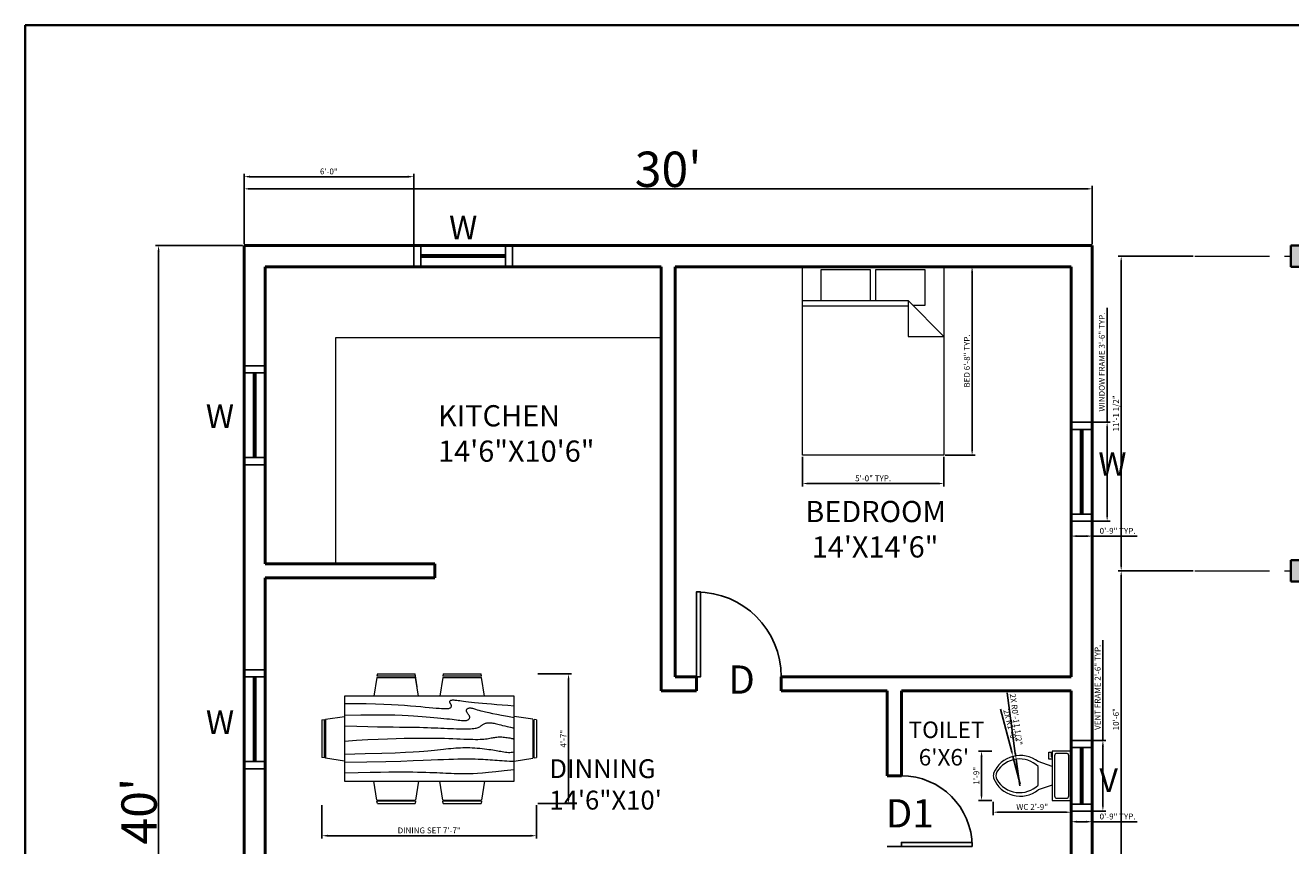
# Model space of a CAD drawing. Units: inches. Extents: x 2150 to 10686, y 1035 to 5077.
# Tile 3 of 12: x 2150 to 2687, y 1753 to 2101. Entities that reach past the tile are written whole.
import ezdxf

# ---------------------------------------------------------------- set-up
doc = ezdxf.new("R2010")
doc.units = ezdxf.units.IN
doc.linetypes.add('CENTER', pattern=[50.8, 31.75, -6.35, 6.35, -6.35])
for name, color, linetype, lineweight in [('A-ANNO-DIMS', 2, 'Continuous', 18), ('A-ANNO-IDEN', 2, 'Continuous', 18), ('A-ANNO-TTLB', 7, 'Continuous', 35), ('A-AREA-IDEN', 7, 'Continuous', 18), ('A-COLS', 7, 'Continuous', 35), ('A-COLS-PATT', 8, 'Continuous', 13), ('A-DOOR', 4, 'Continuous', 25), ('A-FLOR-FIXT', 9, 'Continuous', 18), ('A-FURN', 8, 'Continuous', 18), ('A-GLAZ', 30, 'Continuous', 25), ('A-GRID', 1, 'CENTER', 18), ('A-WALL', 18, 'Continuous', 50)]:
    doc.layers.add(name, color=color, linetype=linetype, lineweight=lineweight)
doc.styles.get("Standard").update_dxf_attribs({"font": 'arial.ttf'})
doc.dimstyles.new('ISO-25', dxfattribs={"dimtxt": 2.5, "dimasz": 2.5, "dimexe": 1.25, "dimexo": 0.625, "dimtad": 1, "dimdec": 0, "dimlunit": 3, "dimtxsty": 'Standard', "dimcen": 2.5, "dimadec": 0, "dimazin": 0, "dimtfac": 1, "dimtdec": 0, "dimtmove": 0, "dimatfit": 3, "dimfxl": 1, "dimarcsym": 0})

# ---------------------------------------------------------------- blocks, each defined once
blk = doc.blocks.new('Bed - Queen')
for p, q in [((0, -80.00003), (0, 0)), ((0, 0), (59.99999, 0)), ((59.99999, 0), (59.99999, -80.00003)), ((7.99999, -1.2), (28.79998, -1.2)), ((7.99999, -14.4), (7.99999, -1.2)), ((28.79998, -1.2), (28.79998, -14.4)), ((31.19999, -1.2), (51.99999, -1.2)), ((31.19999, -14.4), (31.19999, -1.2)), ((51.99999, -1.2), (51.99999, -16.4)), ((0, -14.4), (44.8, -14.4)), ((59.99999, -29.6), (44.8, -14.4)), ((44.8, -14.4), (44.8, -29.6)), ((44.8, -16.8), (0, -16.8)), ((51.99999, -16.4), (46.79936, -16.4)), ((44.8, -29.6), (59.99999, -29.6)), ((59.99999, -80.00003), (0, -80.00003))]:
    blk.add_line(p, q)
blk = doc.blocks.new('Dining Set - 36 x 72 in.')
for p, q in [((-22, 27.5), (-22.1562, 26.50042)), ((-22, 27.5), (-6, 27.5)), ((-5.14035, 21.99844), (-6, 27.5)), ((6, 27.5), (5.8438, 26.50042)), ((6, 27.5), (22, 27.5)), ((22.1563, 26.49966), (22, 27.5)), ((-22.2343, 26.00059), (-23.4847, 17.99762)), ((-22.2304, 26), (-5.7608, 26)), ((-5.8416, 26.5), (-22.1534, 26.5)), ((-4.5152, 17.99762), (-5.7655, 25.99926)), ((5.7657, 26.00059), (4.5153, 17.99762)), ((5.7696, 26), (22.2392, 26)), ((22.1584, 26.5), (5.8466, 26.5)), ((23.4848, 17.99762), (22.2345, 25.99926)), ((36, 18), (-36, 18)), ((-36, 18), (-36, -18)), ((36, -18), (36, 18)), ((-45.5, 8), (-44.5004, 8.15617)), ((-45.5, 8), (-45.5, -8)), ((-44.5, -8.15843), (-44.5, 8.15338)), ((-44.0006, 8.23428), (-35.9976, 9.48474)), ((-44, 8.23041), (-44, -8.23915)), ((44.0006, 8.23428), (35.9976, 9.48474)), ((44, 8.23041), (44, -8.23915)), ((44.5, -8.15843), (44.5, 8.15338)), ((45.5, 8), (44.5005, 8.15617)), ((45.5, 8), (45.5, -8)), ((-44.4997, -8.15631), (-45.5, -8)), ((-35.9976, -9.48476), (-43.9993, -8.2345)), ((35.9976, -9.48476), (43.9993, -8.2345)), ((44.4997, -8.15631), (45.5, -8)), ((-36, -18), (36, -18)), ((-22.2343, -26.0006), (-23.4847, -17.99762)), ((-4.5152, -17.99762), (-5.7655, -25.99928)), ((5.7657, -26.0006), (4.5153, -17.99762)), ((23.4848, -17.99762), (22.2345, -25.99928)), ((-22.2304, -26), (-5.7608, -26)), ((-22, -27.5), (-22.1562, -26.50044)), ((-5.8416, -26.5), (-22.1534, -26.5)), ((-5.8437, -26.49967), (-6, -27.5)), ((5.7696, -26), (22.2392, -26)), ((6, -27.5), (5.8438, -26.50044)), ((22.1584, -26.5), (5.8466, -26.5)), ((22.1563, -26.49967), (22, -27.5)), ((-22, -27.5), (-6, -27.5)), ((6, -27.5), (22, -27.5))]:
    blk.add_line(p, q)
for points in [[(-36, 15), (-31.1772, 14.97754), (-26.8079, 14.91406), (-22.8538, 14.81543), (-19.276, 14.6875), (-16.0362, 14.53613), (-13.0957, 14.36718), (-10.4159, 14.18652), (-7.9583, 14), (-5.6904, 13.81315), (-3.6035, 13.63021), (-1.6954, 13.45508), (0.0365, 13.29166), (1.5945, 13.14388), (2.9811, 13.01562), (4.1988, 12.9108), (5.25, 12.83333), (6.1393, 12.78613), (6.8802, 12.76823), (7.4883, 12.77767), (7.9792, 12.8125), (8.3685, 12.87077), (8.6719, 12.95052), (8.9049, 13.0498), (9.0833, 13.16666), (9.2205, 13.29899), (9.3216, 13.44401), (9.3895, 13.59879), (9.4271, 13.76041), (9.4373, 13.92594), (9.4232, 14.09245), (9.3875, 14.257), (9.3333, 14.41666), (9.2638, 14.56917), (9.1836, 14.71484), (9.0975, 14.85465), (9.0104, 14.98958), (8.9272, 15.1206), (8.8529, 15.2487), (8.7922, 15.37483), (8.75, 15.5), (8.7305, 15.62467), (8.7344, 15.74739), (8.7617, 15.86621), (8.8125, 15.97916), (8.8867, 16.08431), (8.9844, 16.17968), (9.1055, 16.26334), (9.25, 16.33333), (9.4189, 16.38802), (9.6172, 16.42708), (9.8506, 16.45052), (10.125, 16.45833), (10.4463, 16.45052), (10.8203, 16.42708), (11.2529, 16.38802), (11.75, 16.33333), (12.3184, 16.26318), (12.9694, 16.17838), (13.7151, 16.07991), (14.5677, 15.96875), (15.5395, 15.84586), (16.6426, 15.71224), (17.8893, 15.56884), (19.2917, 15.41666), (20.859, 15.25667), (22.5879, 15.08984), (24.4721, 14.91715), (26.5052, 14.73958), (28.6809, 14.5581), (30.9929, 14.3737), (33.4347, 14.18733), (36, 14)], [(-36, 10), (-28.9766, 10.14274), (-23.1725, 10.20442), (-18.4241, 10.19775), (-14.5677, 10.13541), (-11.4399, 10.03011), (-8.877, 9.89453), (-6.7154, 9.74137), (-4.7917, 9.58333), (-2.9698, 9.43082), (-1.2246, 9.28515), (0.4415, 9.14534), (2.026, 9.01041), (3.5266, 8.87939), (4.9408, 8.7513), (6.266, 8.62516), (7.5, 8.5), (8.6411, 8.37549), (9.6914, 8.2539), (10.6538, 8.13818), (11.5312, 8.03125), (12.3267, 7.93603), (13.043, 7.85547), (13.6831, 7.79248), (14.25, 7.75), (14.7471, 7.7303), (15.1797, 7.73307), (15.5537, 7.75732), (15.875, 7.80208), (16.1494, 7.86637), (16.3828, 7.94922), (16.5811, 8.04964), (16.75, 8.16666), (16.8944, 8.29915), (17.0143, 8.44531), (17.1089, 8.60319), (17.1771, 8.77083), (17.218, 8.94629), (17.2305, 9.1276), (17.2137, 9.31282), (17.1667, 9.5), (17.0895, 9.6875), (16.987, 9.875), (16.8649, 10.0625), (16.7292, 10.25), (16.5856, 10.4375), (16.4401, 10.625), (16.2985, 10.8125), (16.1667, 11), (16.05, 11.18733), (15.9518, 11.3737), (15.8752, 11.5581), (15.8229, 11.73958), (15.798, 11.91715), (15.8034, 12.08984), (15.842, 12.25667), (15.9167, 12.41666), (16.0295, 12.56836), (16.1784, 12.70833), (16.3605, 12.83268), (16.5729, 12.9375), (16.8127, 13.01888), (17.0768, 13.07291), (17.3625, 13.0957), (17.6667, 13.08333), (17.9894, 13.03312), (18.3418, 12.94726), (18.7382, 12.82918), (19.1927, 12.68229), (19.7195, 12.51001), (20.3327, 12.31575), (21.0465, 12.10294), (21.875, 11.875), (22.8357, 11.63354), (23.959, 11.37304), (25.2786, 11.08618), (26.8282, 10.76562), (28.6414, 10.40405), (30.752, 9.99414), (33.1936, 9.52856), (36, 9)], [(-36, 5.5), (-30.7157, 5.3348), (-26.069, 5.20963), (-21.9946, 5.11767), (-18.4271, 5.05208), (-15.3009, 5.00602), (-12.5508, 4.97265), (-10.1112, 4.94515), (-7.9167, 4.91666), (-5.909, 4.88167), (-4.0586, 4.83984), (-2.3429, 4.79215), (-0.7396, 4.73958), (0.7739, 4.6831), (2.22, 4.6237), (3.6213, 4.56233), (5, 4.5), (6.373, 4.43782), (7.7344, 4.3776), (9.0723, 4.32129), (10.375, 4.27083), (11.6309, 4.22819), (12.8281, 4.19531), (13.9551, 4.17415), (15, 4.16666), (15.954, 4.17448), (16.819, 4.19791), (17.6001, 4.23698), (18.3021, 4.29166), (18.9299, 4.36198), (19.4883, 4.44791), (19.9823, 4.54948), (20.4167, 4.66666), (20.7969, 4.79899), (21.1302, 4.94401), (21.4245, 5.09879), (21.6875, 5.26041), (21.9271, 5.42594), (22.1511, 5.59245), (22.3672, 5.757), (22.5834, 5.91666), (22.8065, 6.06868), (23.0404, 6.21093), (23.2879, 6.34147), (23.5521, 6.45833), (23.8358, 6.55957), (24.142, 6.64323), (24.4735, 6.70735), (24.8334, 6.75), (25.2235, 6.76969), (25.642, 6.76692), (26.0858, 6.74267), (26.5521, 6.69791), (27.0379, 6.63362), (27.5404, 6.55078), (28.0565, 6.45036), (28.5834, 6.33333), (29.1242, 6.19987), (29.7071, 6.04687), (30.3661, 5.87044), (31.1354, 5.66666), (32.0493, 5.43164), (33.142, 5.16146), (34.4475, 4.85221), (36, 4.5)], [(-36, -1), (-30.7915, -0.6591), (-26.0195, -0.38216), (-21.6519, -0.16284), (-17.6563, 0.00521), (-14.0005, 0.12833), (-10.6523, 0.21289), (-7.5796, 0.26522), (-4.75, 0.29166), (-2.134, 0.29793), (0.2878, 0.28711), (2.5317, 0.26163), (4.6146, 0.22396), (6.5529, 0.17651), (8.3633, 0.12174), (10.0623, 0.06209), (11.6667, 0), (13.1899, -0.06201), (14.6341, -0.1211), (15.9982, -0.17432), (17.2813, -0.21875), (18.4823, -0.25147), (19.6003, -0.26953), (20.6343, -0.27002), (21.5834, -0.25), (22.4481, -0.20768), (23.2357, -0.14584), (23.9549, -0.06836), (24.6146, 0.02083), (25.2235, 0.11784), (25.7904, 0.21875), (26.3241, 0.31966), (26.8334, 0.41666), (27.3265, 0.50618), (27.8099, 0.58593), (28.2894, 0.65397), (28.7709, 0.70833), (29.2601, 0.74707), (29.763, 0.76823), (30.2855, 0.76985), (30.8334, 0.75), (31.4088, 0.70784), (31.9994, 0.64713), (32.589, 0.57275), (33.1615, 0.48958), (33.7008, 0.4025), (34.1908, 0.3164), (34.6153, 0.23616), (34.9584, 0.16666), (35.2099, 0.11165), (35.3848, 0.07031), (35.504, 0.04069), (35.5886, 0.02083), (35.6594, 0.00879), (35.7377, 0.0026), (35.8442, 0.00032), (36, 0)], [(-36, -6.5), (-27.1843, -6.31267), (-20.084, -6.1263), (-14.469, -5.9419), (-10.1094, -5.76042), (-6.7752, -5.58285), (-4.2363, -5.41016), (-2.2629, -5.24333), (-0.625, -5.08334), (0.8708, -4.93099), (2.2715, -4.78646), (3.5872, -4.64974), (4.8281, -4.52084), (6.0046, -4.39974), (7.127, -4.28646), (8.2053, -4.18099), (9.25, -4.08334), (10.2705, -3.99382), (11.2734, -3.91407), (12.2647, -3.84603), (13.25, -3.79167), (14.2354, -3.75293), (15.2266, -3.73177), (16.2295, -3.73015), (17.25, -3.75), (18.2912, -3.79248), (19.3451, -3.85547), (20.4009, -3.93604), (21.4479, -4.03125), (22.4754, -4.13819), (23.4727, -4.25391), (24.4289, -4.37549), (25.3334, -4.5), (26.1785, -4.62492), (26.9694, -4.74935), (27.7145, -4.87281), (28.4219, -4.99479), (29.1, -5.11483), (29.7572, -5.23242), (30.4016, -5.34709), (31.0417, -5.45834), (31.6837, -5.56437), (32.3262, -5.65821), (32.9658, -5.73153), (33.599, -5.77604), (34.2224, -5.78345), (34.8327, -5.74545), (35.4264, -5.65373), (36, -5.5)], [(-36, -10), (-26.4022, -9.81299), (-18.4675, -9.62891), (-11.9839, -9.45069), (-6.7396, -9.28125), (-2.5226, -9.12354), (0.8789, -8.98047), (3.6769, -8.85498), (6.0833, -8.75), (8.2767, -8.66765), (10.3021, -8.60677), (12.1712, -8.56543), (13.8958, -8.54167), (15.4876, -8.53353), (16.9583, -8.53907), (18.3197, -8.55632), (19.5834, -8.58334), (20.7616, -8.61841), (21.8685, -8.66081), (22.9188, -8.71004), (23.9271, -8.76563), (24.9081, -8.82707), (25.8763, -8.89388), (26.8465, -8.96558), (27.8334, -9.04167), (28.8474, -9.12118), (29.8828, -9.20117), (30.93, -9.27824), (31.9792, -9.34896), (33.0205, -9.40991), (34.0443, -9.45768), (35.0407, -9.48885), (36, -9.5)], [(-36, -14.5), (-30.0881, -14.33513), (-25.0332, -14.21224), (-20.7312, -14.12647), (-17.0781, -14.07292), (-13.97, -14.04671), (-11.3027, -14.04297), (-8.9724, -14.05681), (-6.875, -14.08334), (-4.9224, -14.11833), (-3.0905, -14.16016), (-1.3709, -14.20785), (0.2448, -14.26042), (1.7647, -14.3169), (3.1973, -14.3763), (4.5507, -14.43767), (5.8333, -14.5), (7.0554, -14.5621), (8.235, -14.62175), (9.3922, -14.67652), (10.5469, -14.72396), (11.7192, -14.76164), (12.929, -14.78711), (14.1965, -14.79794), (15.5417, -14.79167), (16.9933, -14.76424), (18.6152, -14.70508), (20.4804, -14.60197), (22.6615, -14.44271), (25.2312, -14.21509), (28.2624, -13.9069), (31.8277, -13.50594), (36, -13)]]:
    blk.add_lwpolyline(points)
blk = doc.blocks.new('Toilet - top')
for p, q in [((9.5, -6), (9.5, -2)), ((-10, -8.5), (-8, -8.5)), ((-10, -9.5), (-10, -8.5)), ((-7, -9.5), (-10, -9.5)), ((-8, -8.5), (-8, -8)), ((-7, -8), (-7, -9.5)), ((-4, -8), (-6, -14)), ((4, -8), (6, -14)), ((4, -14), (-4, -14))]:
    blk.add_line(p, q)
blk.add_lwpolyline([(10.5, -8), (10.5, 0), (-10.5, 0), (-10.5, -8)], close=True)
for points in [[(-9.5, -2), (-9.5, -6)], [(8.5, -1), (-8.5, -1)], [(-8.5, -7), (8.5, -7)]]:
    blk.add_lwpolyline(points)
for centre, radius, start, end in [((-8.62, -1.88), 0.884, 81.8699, 188.1301), ((8.62, -1.88), 0.884, 351.8699, 98.1301), ((-8.62, -6.12), 0.884, 171.8699, 278.1301), ((8.62, -6.12), 0.884, 261.8699, 8.1301), ((3.52, -21.58), 12.17, 141.4691, 247.9714), ((4.2, -21.82), 11.33, 136.3677, 238.9468), ((-3.52, -21.58), 12.17, 292.0284, 38.5307), ((-4.2, -21.82), 11.33, 301.053, 43.6321), ((0, -27.88), 4, 245.7318, 294.2682), ((0, -29), 4, 254.8605, 285.1395)]:
    blk.add_arc(centre, radius, start, end)
blk = doc.blocks.new('*U8')
for p, q in [((0, 0), (0, -6)), ((36, 0), (36, -6))]:
    blk.add_line(p, q)
blk.add_lwpolyline([(0, 0), (0, 36), (1.75, 36), (1.75, 0)], close=True)
blk.add_arc((0, 0), 36, 0, 90)
blk = doc.blocks.new('*U10')
for p, q in [((-30, 0), (-30, -6)), ((0, 0), (0, -6))]:
    blk.add_line(p, q)
blk.add_lwpolyline([(0, 0), (0, 30), (-1.75, 30), (-1.75, 0)], close=True)
blk.add_arc((0, 0), 30, 90, 180)
blk = doc.blocks.new('*D12')
at = {"layer": 'A-ANNO-DIMS', "color": 0, "lineweight": -2, "transparency": 16777216}
for p, q in [((2242.69, 2007.92), (2242.69, 2032.59)), ((2245.19, 2031.34), (2600.19, 2031.34)), ((2602.69, 2007.92), (2602.69, 2032.59))]:
    blk.add_line(p, q, dxfattribs=at)
at = {"layer": 'A-ANNO-DIMS', "color": 0, "transparency": 16777216}
for points in [[(2245.19, 2031.76), (2245.19, 2030.92), (2242.69, 2031.34)], [(2600.19, 2031.76), (2600.19, 2030.92), (2602.69, 2031.34)]]:
    blk.add_solid(points, dxfattribs=at)
at = {"layer": 'Defpoints', "color": 0, "transparency": 16777216}
for p in [(2602.69, 2031.34), (2242.69, 2007.29), (2602.69, 2007.29)]:
    blk.add_point(p, dxfattribs=at)
at = {"layer": 'A-ANNO-DIMS', "color": 0, "transparency": 16777216, "insert": (2422.69, 2039.63), "char_height": 2.5, "attachment_point": 5}
blk.add_mtext("{\\H6x;30'}", dxfattribs=at)
blk = doc.blocks.new('*D13')
at = {"layer": 'A-ANNO-DIMS', "color": 0, "lineweight": -2, "transparency": 16777216}
for p, q in [((2242.07, 2007.29), (2205.18, 2007.29)), ((2206.43, 2004.79), (2206.43, 1529.79)), ((2242.07, 1527.29), (2205.18, 1527.29))]:
    blk.add_line(p, q, dxfattribs=at)
at = {"layer": 'A-ANNO-DIMS', "color": 0, "transparency": 16777216}
for points in [[(2206.01, 2004.79), (2206.85, 2004.79), (2206.43, 2007.29)], [(2206.01, 1529.79), (2206.85, 1529.79), (2206.43, 1527.29)]]:
    blk.add_solid(points, dxfattribs=at)
at = {"layer": 'Defpoints', "color": 0, "transparency": 16777216}
for p in [(2242.69, 2007.29), (2206.43, 1527.29), (2242.69, 1527.29)]:
    blk.add_point(p, dxfattribs=at)
at = {"layer": 'A-ANNO-DIMS', "color": 0, "transparency": 16777216, "insert": (2198.15, 1767.29), "char_height": 2.5, "attachment_point": 5, "rotation": 90}
blk.add_mtext("{\\H6x;40'}", dxfattribs=at)
blk = doc.blocks.new('COL-SQUARE-9IN')
for p, q in [((0, 9), (9, 9)), ((0, 0), (0, 9)), ((9, 9), (9, 0)), ((9, 0), (0, 0))]:
    blk.add_line(p, q)
blk = doc.blocks.new('WINDOW-36IN')
for p, q in [((9, 42), (0, 42)), ((9, 39), (0, 39)), ((4, 39), (4, 3)), ((4.5, 39), (4.5, 3)), ((5, 39), (5, 3)), ((9, 3), (0, 3)), ((9, 0), (0, 0))]:
    blk.add_line(p, q)
blk = doc.blocks.new('VENT-24IN')
for p, q in [((0, 30), (9, 30)), ((0, 27), (9, 27)), ((4, 27), (4, 3)), ((4.5, 27), (4.5, 3)), ((5, 27), (5, 3)), ((0, 3), (9, 3)), ((0, 0), (9, 0))]:
    blk.add_line(p, q)
blk = doc.blocks.new('*D40')
at = {"layer": 'A-ANNO-DIMS', "color": 0, "lineweight": -2, "transparency": 16777216}
for p, q in [((2540.32, 1998.29), (2552.94, 1998.29)), ((2551.69, 1920.79), (2551.69, 1995.79)), ((2540.32, 1918.29), (2552.94, 1918.29))]:
    blk.add_line(p, q, dxfattribs=at)
at = {"layer": 'A-ANNO-DIMS', "color": 0, "transparency": 16777216}
for points in [[(2551.28, 1995.79), (2552.11, 1995.79), (2551.69, 1998.29)], [(2551.28, 1920.79), (2552.11, 1920.79), (2551.69, 1918.29)]]:
    blk.add_solid(points, dxfattribs=at)
at = {"layer": 'Defpoints', "color": 0, "transparency": 16777216}
for p in [(2539.69, 1998.29), (2551.69, 1998.29), (2539.69, 1918.29)]:
    blk.add_point(p, dxfattribs=at)
at = {"layer": 'A-ANNO-DIMS', "color": 0, "transparency": 16777216, "insert": (2549.79, 1958.29), "char_height": 2.5, "attachment_point": 5, "rotation": 90}
blk.add_mtext('BED 6\'-8" TYP.', dxfattribs=at)
blk = doc.blocks.new('*D41')
at = {"layer": 'A-ANNO-DIMS', "color": 0, "lineweight": -2, "transparency": 16777216}
for p, q in [((2479.69, 1917.67), (2479.69, 1905.04)), ((2539.69, 1917.67), (2539.69, 1905.04)), ((2482.19, 1906.29), (2537.19, 1906.29))]:
    blk.add_line(p, q, dxfattribs=at)
at = {"layer": 'A-ANNO-DIMS', "color": 0, "transparency": 16777216}
for points in [[(2482.19, 1906.71), (2482.19, 1905.87), (2479.69, 1906.29)], [(2537.19, 1906.71), (2537.19, 1905.87), (2539.69, 1906.29)]]:
    blk.add_solid(points, dxfattribs=at)
at = {"layer": 'Defpoints', "color": 0, "transparency": 16777216}
for p in [(2479.69, 1918.29), (2539.69, 1918.29), (2539.69, 1906.29)]:
    blk.add_point(p, dxfattribs=at)
at = {"layer": 'A-ANNO-DIMS', "color": 0, "transparency": 16777216, "insert": (2509.69, 1908.19), "char_height": 2.5, "attachment_point": 5}
blk.add_mtext('5\'-0" TYP.', dxfattribs=at)
blk = doc.blocks.new('*D44')
at = {"layer": 'A-ANNO-DIMS', "color": 0, "lineweight": -2, "transparency": 16777216}
for p, q in [((2608.99, 1932.29), (2608.99, 1980.87)), ((2603.32, 1932.29), (2610.24, 1932.29)), ((2608.99, 1892.79), (2608.99, 1929.79)), ((2603.32, 1890.29), (2610.24, 1890.29))]:
    blk.add_line(p, q, dxfattribs=at)
at = {"layer": 'A-ANNO-DIMS', "color": 0, "transparency": 16777216}
for points in [[(2608.58, 1929.79), (2609.41, 1929.79), (2608.99, 1932.29)], [(2608.58, 1892.79), (2609.41, 1892.79), (2608.99, 1890.29)]]:
    blk.add_solid(points, dxfattribs=at)
at = {"layer": 'Defpoints', "color": 0, "transparency": 16777216}
for p in [(2602.69, 1932.29), (2608.99, 1932.29), (2602.69, 1890.29)]:
    blk.add_point(p, dxfattribs=at)
at = {"layer": 'A-ANNO-DIMS', "color": 0, "transparency": 16777216, "insert": (2607.07, 1957.83), "char_height": 2.5, "attachment_point": 5, "rotation": 90}
blk.add_mtext('WINDOW FRAME 3\'-6" TYP.', dxfattribs=at)
blk = doc.blocks.new('*D45')
at = {"layer": 'A-ANNO-DIMS', "color": 0, "lineweight": -2, "transparency": 16777216}
for p, q in [((2593.69, 1889.67), (2593.69, 1882.74)), ((2602.69, 1889.67), (2602.69, 1882.74)), ((2596.19, 1883.99), (2600.19, 1883.99)), ((2602.69, 1883.99), (2621.68, 1883.99))]:
    blk.add_line(p, q, dxfattribs=at)
at = {"layer": 'A-ANNO-DIMS', "color": 0, "transparency": 16777216}
for points in [[(2596.19, 1884.41), (2596.19, 1883.57), (2593.69, 1883.99)], [(2600.19, 1884.41), (2600.19, 1883.57), (2602.69, 1883.99)]]:
    blk.add_solid(points, dxfattribs=at)
at = {"layer": 'Defpoints', "color": 0, "transparency": 16777216}
for p in [(2593.69, 1890.29), (2602.69, 1890.29), (2602.69, 1883.99)]:
    blk.add_point(p, dxfattribs=at)
at = {"layer": 'A-ANNO-DIMS', "color": 0, "transparency": 16777216, "insert": (2613.44, 1885.89), "char_height": 2.5, "attachment_point": 5}
blk.add_mtext('0\'-9" TYP.', dxfattribs=at)
blk = doc.blocks.new('*D46')
at = {"layer": 'A-ANNO-DIMS', "color": 0, "lineweight": -2, "transparency": 16777216}
for p, q in [((2607.19, 1797.29), (2607.19, 1839.89)), ((2603.32, 1797.29), (2608.44, 1797.29)), ((2607.19, 1769.79), (2607.19, 1794.79)), ((2603.32, 1767.29), (2608.44, 1767.29))]:
    blk.add_line(p, q, dxfattribs=at)
at = {"layer": 'A-ANNO-DIMS', "color": 0, "transparency": 16777216}
for points in [[(2606.78, 1794.79), (2607.61, 1794.79), (2607.19, 1797.29)], [(2606.78, 1769.79), (2607.61, 1769.79), (2607.19, 1767.29)]]:
    blk.add_solid(points, dxfattribs=at)
at = {"layer": 'Defpoints', "color": 0, "transparency": 16777216}
for p in [(2602.69, 1797.29), (2607.19, 1797.29), (2602.69, 1767.29)]:
    blk.add_point(p, dxfattribs=at)
at = {"layer": 'A-ANNO-DIMS', "color": 0, "transparency": 16777216, "insert": (2605.29, 1819.84), "char_height": 2.5, "attachment_point": 5, "rotation": 90}
blk.add_mtext('VENT FRAME 2\'-6" TYP.', dxfattribs=at)
blk = doc.blocks.new('*D47')
at = {"layer": 'A-ANNO-DIMS', "color": 0, "lineweight": -2, "transparency": 16777216}
for p, q in [((2593.69, 1766.67), (2593.69, 1761.54)), ((2596.19, 1762.79), (2600.19, 1762.79)), ((2602.69, 1766.67), (2602.69, 1761.54)), ((2602.69, 1762.79), (2621.68, 1762.79))]:
    blk.add_line(p, q, dxfattribs=at)
at = {"layer": 'A-ANNO-DIMS', "color": 0, "transparency": 16777216}
for points in [[(2596.19, 1763.21), (2596.19, 1762.37), (2593.69, 1762.79)], [(2600.19, 1763.21), (2600.19, 1762.37), (2602.69, 1762.79)]]:
    blk.add_solid(points, dxfattribs=at)
at = {"layer": 'Defpoints', "color": 0, "transparency": 16777216}
for p in [(2593.69, 1767.29), (2602.69, 1767.29), (2602.69, 1762.79)]:
    blk.add_point(p, dxfattribs=at)
at = {"layer": 'A-ANNO-DIMS', "color": 0, "transparency": 16777216, "insert": (2613.44, 1764.69), "char_height": 2.5, "attachment_point": 5}
blk.add_mtext('0\'-9" TYP.', dxfattribs=at)
blk = doc.blocks.new('*D54')
at = {"layer": 'A-ANNO-DIMS', "color": 0, "lineweight": -2, "transparency": 16777216}
for p, q in [((2560.65, 1771.17), (2560.65, 1765.58)), ((2593.69, 1771.17), (2593.69, 1765.58)), ((2563.15, 1766.83), (2591.19, 1766.83))]:
    blk.add_line(p, q, dxfattribs=at)
at = {"layer": 'A-ANNO-DIMS', "color": 0, "transparency": 16777216}
for points in [[(2563.15, 1767.25), (2563.15, 1766.42), (2560.65, 1766.83)], [(2591.19, 1767.25), (2591.19, 1766.42), (2593.69, 1766.83)]]:
    blk.add_solid(points, dxfattribs=at)
at = {"layer": 'Defpoints', "color": 0, "transparency": 16777216}
for p in [(2560.65, 1771.79), (2593.69, 1771.79), (2593.69, 1766.83)]:
    blk.add_point(p, dxfattribs=at)
at = {"layer": 'A-ANNO-DIMS', "color": 0, "transparency": 16777216, "insert": (2577.17, 1768.75), "char_height": 2.5, "attachment_point": 5}
blk.add_mtext('WC 2\'-9"', dxfattribs=at)
blk = doc.blocks.new('*D55')
at = {"layer": 'A-ANNO-DIMS', "color": 0, "lineweight": -2, "transparency": 16777216}
for p, q in [((2560.02, 1792.79), (2554.44, 1792.79)), ((2555.69, 1790.29), (2555.69, 1774.29)), ((2560.02, 1771.79), (2554.44, 1771.79))]:
    blk.add_line(p, q, dxfattribs=at)
at = {"layer": 'A-ANNO-DIMS', "color": 0, "transparency": 16777216}
for points in [[(2555.27, 1790.29), (2556.11, 1790.29), (2555.69, 1792.79)], [(2555.27, 1774.29), (2556.11, 1774.29), (2555.69, 1771.79)]]:
    blk.add_solid(points, dxfattribs=at)
at = {"layer": 'Defpoints', "color": 0, "transparency": 16777216}
for p in [(2560.65, 1792.79), (2555.69, 1771.79), (2560.65, 1771.79)]:
    blk.add_point(p, dxfattribs=at)
at = {"layer": 'A-ANNO-DIMS', "color": 0, "transparency": 16777216, "insert": (2553.79, 1782.29), "char_height": 2.5, "attachment_point": 5, "rotation": 90}
blk.add_mtext('1\'-9"', dxfattribs=at)
blk = doc.blocks.new('*D56')
at = {"layer": 'A-ANNO-DIMS', "color": 0, "lineweight": -2, "transparency": 16777216}
for p, q in [((2275.77, 1769.89), (2275.77, 1755.61)), ((2366.77, 1769.89), (2366.77, 1755.61)), ((2278.27, 1756.86), (2364.27, 1756.86))]:
    blk.add_line(p, q, dxfattribs=at)
at = {"layer": 'A-ANNO-DIMS', "color": 0, "transparency": 16777216}
for points in [[(2278.27, 1757.28), (2278.27, 1756.44), (2275.77, 1756.86)], [(2364.27, 1757.28), (2364.27, 1756.44), (2366.77, 1756.86)]]:
    blk.add_solid(points, dxfattribs=at)
at = {"layer": 'Defpoints', "color": 0, "transparency": 16777216}
for p in [(2275.77, 1770.51), (2366.77, 1770.51), (2366.77, 1756.86)]:
    blk.add_point(p, dxfattribs=at)
at = {"layer": 'A-ANNO-DIMS', "color": 0, "transparency": 16777216, "insert": (2321.27, 1758.78), "char_height": 2.5, "attachment_point": 5}
blk.add_mtext('DINING SET 7\'-7"', dxfattribs=at)
blk = doc.blocks.new('*D57')
at = {"layer": 'A-ANNO-DIMS', "color": 0, "lineweight": -2, "transparency": 16777216}
for p, q in [((2367.39, 1825.51), (2381.67, 1825.51)), ((2380.42, 1773.01), (2380.42, 1823.01)), ((2367.39, 1770.51), (2381.67, 1770.51))]:
    blk.add_line(p, q, dxfattribs=at)
at = {"layer": 'A-ANNO-DIMS', "color": 0, "transparency": 16777216}
for points in [[(2380, 1823.01), (2380.84, 1823.01), (2380.42, 1825.51)], [(2380, 1773.01), (2380.84, 1773.01), (2380.42, 1770.51)]]:
    blk.add_solid(points, dxfattribs=at)
at = {"layer": 'Defpoints', "color": 0, "transparency": 16777216}
for p in [(2366.77, 1825.51), (2380.42, 1825.51), (2366.77, 1770.51)]:
    blk.add_point(p, dxfattribs=at)
at = {"layer": 'A-ANNO-DIMS', "color": 0, "transparency": 16777216, "insert": (2378.54, 1798.01), "char_height": 2.5, "attachment_point": 5, "rotation": 90}
blk.add_mtext('4\'-7"', dxfattribs=at)
blk = doc.blocks.new('*D80')
at = {"layer": 'A-ANNO-DIMS', "color": 0, "lineweight": -2, "transparency": 16777216}
for p, q in [((2645.54, 2002.79), (2613.71, 2002.79)), ((2614.96, 2000.29), (2614.96, 1871.79)), ((2645.54, 1869.29), (2613.71, 1869.29))]:
    blk.add_line(p, q, dxfattribs=at)
at = {"layer": 'A-ANNO-DIMS', "color": 0, "transparency": 16777216}
for points in [[(2614.55, 2000.29), (2615.38, 2000.29), (2614.96, 2002.79)], [(2614.55, 1871.79), (2615.38, 1871.79), (2614.96, 1869.29)]]:
    blk.add_solid(points, dxfattribs=at)
at = {"layer": 'Defpoints', "color": 0, "transparency": 16777216}
for p in [(2646.16, 2002.79), (2614.96, 1869.29), (2646.16, 1869.29)]:
    blk.add_point(p, dxfattribs=at)
at = {"layer": 'A-ANNO-DIMS', "color": 0, "transparency": 16777216, "insert": (2613.05, 1936.04), "char_height": 2.5, "attachment_point": 5, "rotation": 90}
blk.add_mtext('11\'-1 1/2"', dxfattribs=at)
blk = doc.blocks.new('*D81')
at = {"layer": 'A-ANNO-DIMS', "color": 0, "lineweight": -2, "transparency": 16777216}
for p, q in [((2645.54, 1869.29), (2613.71, 1869.29)), ((2614.96, 1866.79), (2614.96, 1745.79)), ((2645.54, 1743.29), (2613.71, 1743.29))]:
    blk.add_line(p, q, dxfattribs=at)
at = {"layer": 'A-ANNO-DIMS', "color": 0, "transparency": 16777216}
for points in [[(2614.55, 1866.79), (2615.38, 1866.79), (2614.96, 1869.29)], [(2614.55, 1745.79), (2615.38, 1745.79), (2614.96, 1743.29)]]:
    blk.add_solid(points, dxfattribs=at)
at = {"layer": 'Defpoints', "color": 0, "transparency": 16777216}
for p in [(2646.16, 1869.29), (2614.96, 1743.29), (2646.16, 1743.29)]:
    blk.add_point(p, dxfattribs=at)
at = {"layer": 'A-ANNO-DIMS', "color": 0, "transparency": 16777216, "insert": (2613.06, 1806.29), "char_height": 2.5, "attachment_point": 5, "rotation": 90}
blk.add_mtext('10\'-6"', dxfattribs=at)
blk = doc.blocks.new('*D138')
at = {"layer": 'A-ANNO-DIMS', "color": 0, "lineweight": -2, "transparency": 16777216}
for p, q in [((2242.69, 2007.92), (2242.69, 2037.74)), ((2245.19, 2036.49), (2312.19, 2036.49)), ((2314.69, 2007.92), (2314.69, 2037.74))]:
    blk.add_line(p, q, dxfattribs=at)
at = {"layer": 'A-ANNO-DIMS', "color": 0, "transparency": 16777216}
for points in [[(2245.19, 2036.91), (2245.19, 2036.07), (2242.69, 2036.49)], [(2312.19, 2036.91), (2312.19, 2036.07), (2314.69, 2036.49)]]:
    blk.add_solid(points, dxfattribs=at)
at = {"layer": 'Defpoints', "color": 0, "transparency": 16777216}
for p in [(2314.69, 2036.49), (2242.69, 2007.29), (2314.69, 2007.29)]:
    blk.add_point(p, dxfattribs=at)
at = {"layer": 'A-ANNO-DIMS', "color": 0, "transparency": 16777216, "insert": (2278.69, 2038.39), "char_height": 2.5, "attachment_point": 5}
blk.add_mtext('6\'-0"', dxfattribs=at)
blk = doc.blocks.new('*D151')
at = {"layer": 'A-ANNO-DIMS', "color": 0, "lineweight": -2, "transparency": 16777216}
for p, q in [((2563.76, 1810.56), (2568.39, 1792.96)), ((2572.11, 1778.77), (2569.02, 1790.54))]:
    blk.add_line(p, q, dxfattribs=at)
at = {"layer": 'A-ANNO-DIMS', "color": 0, "transparency": 16777216}
blk.add_solid([(2568.79, 1793.07), (2567.98, 1792.85), (2569.02, 1790.54)], dxfattribs=at)
at = {"layer": 'Defpoints', "color": 0, "transparency": 16777216}
for p in [(2569.02, 1790.54), (2572.11, 1778.77)]:
    blk.add_point(p, dxfattribs=at)
at = {"layer": 'A-ANNO-DIMS', "color": 0, "transparency": 16777216, "insert": (2567.59, 1803.45), "char_height": 2.5, "attachment_point": 5, "rotation": 284.7226}
blk.add_mtext('2X R1\'-0"', dxfattribs=at)
blk = doc.blocks.new('*D152')
at = {"layer": 'A-ANNO-DIMS', "color": 0, "lineweight": -2, "transparency": 16777216}
for p, q in [((2566.57, 1817.54), (2570.03, 1791.8)), ((2571.88, 1778.09), (2570.37, 1789.32))]:
    blk.add_line(p, q, dxfattribs=at)
at = {"layer": 'A-ANNO-DIMS', "color": 0, "transparency": 16777216}
blk.add_solid([(2570.45, 1791.85), (2569.62, 1791.74), (2570.37, 1789.32)], dxfattribs=at)
at = {"layer": 'Defpoints', "color": 0, "transparency": 16777216}
for p in [(2570.37, 1789.32), (2571.88, 1778.09)]:
    blk.add_point(p, dxfattribs=at)
at = {"layer": 'A-ANNO-DIMS', "color": 0, "transparency": 16777216, "insert": (2570.04, 1806.16), "char_height": 2.5, "attachment_point": 5, "rotation": 277.658}
blk.add_mtext('2X R0\'-11 1/2"', dxfattribs=at)

msp = doc.modelspace()

# ---------------------------------------------------------------- hatches: boundary and pattern name
at = {"layer": 'A-COLS-PATT'}
h = msp.add_hatch(color=256, dxfattribs=at)
h.dxf.hatch_style = 1
h.paths.add_polyline_path([(2695.9, 2007.29), (2686.9, 2007.29), (2686.9, 1998.29), (2695.9, 1998.29)])
h.paths.add_polyline_path([(2871.4, 2007.29), (2862.4, 2007.29), (2862.4, 1998.29), (2871.4, 1998.29)])
h.paths.add_polyline_path([(3046.9, 2007.29), (3037.9, 2007.29), (3037.9, 1998.29), (3046.9, 1998.29)])
h.paths.add_polyline_path([(2695.9, 1873.79), (2686.9, 1873.79), (2686.9, 1864.79), (2695.9, 1864.79)])
h.paths.add_polyline_path([(2871.4, 1873.79), (2862.4, 1873.79), (2862.4, 1864.79), (2871.4, 1864.79)])
h.paths.add_polyline_path([(3046.9, 1873.79), (3037.9, 1873.79), (3037.9, 1864.79), (3046.9, 1864.79)])
h.paths.add_polyline_path([(2695.9, 1747.79), (2686.9, 1747.79), (2686.9, 1738.79), (2695.9, 1738.79)])
h.paths.add_polyline_path([(2871.4, 1747.79), (2862.4, 1747.79), (2862.4, 1738.79), (2871.4, 1738.79)])
h.paths.add_polyline_path([(3046.9, 1747.79), (3037.9, 1747.79), (3037.9, 1738.79), (3046.9, 1738.79)])
h.paths.add_polyline_path([(2695.9, 1621.79), (2686.9, 1621.79), (2686.9, 1612.79), (2695.9, 1612.79)])
h.paths.add_polyline_path([(2871.4, 1621.79), (2862.4, 1621.79), (2862.4, 1612.79), (2871.4, 1612.79)])
h.paths.add_polyline_path([(3046.9, 1621.79), (3037.9, 1621.79), (3037.9, 1612.79), (3046.9, 1612.79)])
h.paths.add_polyline_path([(2695.9, 1536.29), (2686.9, 1536.29), (2686.9, 1527.29), (2695.9, 1527.29)])
h.paths.add_polyline_path([(2871.4, 1536.29), (2862.4, 1536.29), (2862.4, 1527.29), (2871.4, 1527.29)])
h.paths.add_polyline_path([(3046.9, 1536.29), (3037.9, 1536.29), (3037.9, 1527.29), (3046.9, 1527.29)])

# ---------------------------------------------------------------- linework, layer by layer
at = {"layer": 'A-ANNO-TTLB'}
msp.add_lwpolyline([(2149.86, 2100.72), (3159.01, 2100.72), (3159.01, 1034.91), (2149.86, 1034.91)], close=True, dxfattribs=at)
at = {"layer": 'A-FLOR-FIXT'}
for p, q in [((2281.69, 1872.29), (2281.69, 1968.29)), ((2281.69, 1968.29), (2419.69, 1968.29))]:
    msp.add_line(p, q, dxfattribs=at)
at = {"layer": 'A-GRID'}
for p, q in [((2646.16, 2002.79), (2686.9, 2002.79)), ((2646.16, 1869.29), (2686.9, 1869.29))]:
    msp.add_line(p, q, dxfattribs=at)
at = {"layer": 'A-WALL'}
for p, q in [((2242.69, 2007.29), (2602.69, 2007.29)), ((2242.69, 1527.29), (2242.69, 2007.29)), ((2602.69, 2007.29), (2602.69, 1527.29)), ((2251.69, 1998.29), (2419.69, 1998.29)), ((2251.69, 1872.29), (2251.69, 1998.29)), ((2419.69, 1818.29), (2419.69, 1998.29)), ((2425.69, 1824.29), (2425.69, 1998.29)), ((2425.69, 1998.29), (2593.69, 1998.29)), ((2593.69, 1998.29), (2593.69, 1824.29)), ((2251.69, 1872.29), (2323.69, 1872.29)), ((2323.69, 1866.29), (2323.69, 1872.29)), ((2251.69, 1866.29), (2323.69, 1866.29)), ((2251.69, 1746.29), (2251.69, 1866.29)), ((2425.69, 1824.29), (2434.69, 1824.29)), ((2434.69, 1818.29), (2434.69, 1824.29)), ((2470.69, 1818.29), (2470.69, 1824.29)), ((2470.69, 1824.29), (2593.69, 1824.29)), ((2419.69, 1818.29), (2434.69, 1818.29)), ((2470.69, 1818.29), (2515.69, 1818.29)), ((2515.69, 1818.29), (2515.69, 1782.29)), ((2521.69, 1818.29), (2521.69, 1782.29)), ((2521.69, 1818.29), (2593.69, 1818.29)), ((2593.69, 1818.29), (2593.69, 1746.29)), ((2515.69, 1782.29), (2521.69, 1782.29))]:
    msp.add_line(p, q, dxfattribs=at)

# ---------------------------------------------------------------- block references
at = {"layer": 'A-COLS'}
for p in [(2686.9, 1998.29), (2686.9, 1864.79)]:
    msp.add_blockref('COL-SQUARE-9IN', p, dxfattribs=at)
at = {"layer": 'A-DOOR'}
msp.add_blockref('*U8', (2434.69, 1824.29), dxfattribs=at)
at = {"layer": 'A-DOOR', "rotation": 270}
msp.add_blockref('*U10', (2521.69, 1752.29), dxfattribs=at)
at = {"layer": 'A-FLOR-FIXT', "rotation": 270}
msp.add_blockref('Toilet - top', (2593.69, 1782.29), dxfattribs=at)
at = {"layer": 'A-FURN'}
for name, p in [('Bed - Queen', (2479.69, 1998.29)), ('Dining Set - 36 x 72 in.', (2321.27, 1798.01))]:
    msp.add_blockref(name, p, dxfattribs=at)
at = {"layer": 'A-GLAZ', "rotation": 269.9999999999994}
msp.add_blockref('WINDOW-36IN', (2314.69, 2007.29), dxfattribs=at)
at = {"layer": 'A-GLAZ'}
for name, p in [('WINDOW-36IN', (2242.69, 1914.29)), ('WINDOW-36IN', (2593.69, 1890.29)), ('WINDOW-36IN', (2242.69, 1785.29)), ('VENT-24IN', (2593.69, 1767.29))]:
    msp.add_blockref(name, p, dxfattribs=at)

# ---------------------------------------------------------------- texts
at = {"layer": 'A-ANNO-IDEN', "attachment_point": 1}
for s, width, insert, char_height in [('W', 198.2229, (2329.72, 2019.89), 10), ('W', 198.2229, (2226.47, 1939.91), 10), ('W', 198.2229, (2605.26, 1919.6), 10), ('D', 907.773, (2448.22, 1829.11), 12), ('W', 198.2229, (2226.51, 1810.03), 10), ('V', 198.2229, (2605.72, 1785.42), 10), ('D1', 907.773, (2515.03, 1772.36), 12)]:
    msp.add_mtext_dynamic_manual_height_columns(s, width=width, gutter_width=12.5, heights=[0], dxfattribs=dict(at, insert=insert, char_height=char_height))
at = {"layer": 'A-AREA-IDEN', "attachment_point": 1}
for s, width, insert, char_height in [('KITCHEN\\P14\'6"X10\'6"', 274.4742, (2325.04, 1939.54), 9), ('BEDROOM\\P 14\'X14\'6"', 318.868, (2480.88, 1898.91), 9), ("TOILET\\P  6'X6'", 287.2446, (2524.77, 1805.31), 7), ('DINNING\\P14\'6"X10\'', 560.271, (2372.25, 1789.3), 8)]:
    msp.add_mtext_dynamic_manual_height_columns(s, width=width, gutter_width=12.5, heights=[0], dxfattribs=dict(at, insert=insert, char_height=char_height))

# ---------------------------------------------------------------- dimensions: what is measured, and where the dimension line sits
at = {"layer": 'A-ANNO-DIMS'}
dim = msp.add_linear_dim(base=(2602.69, 2031.34), p1=(2242.69, 2007.29), p2=(2602.69, 2007.29), text='{\\H6x;<>}', dimstyle='ISO-25', override={"dimclrd": 0, "dimclre": 0, "dimclrt": 0}, dxfattribs=at)
dim.commit()
dim.dimension.update_dxf_attribs({"geometry": '*D12', "text_midpoint": (2422.69, 2031.34), "dimtype": 160})
dim = msp.add_linear_dim(base=(2314.69, 2036.49), p1=(2242.69, 2007.29), p2=(2314.69, 2007.29), dimstyle='ISO-25', override={"dimdec": 1, "dimlfac": 1, "dimrnd": 0, "dimzin": 1, "dimdsep": 46, "dimlunit": 4, "dimfrac": 2}, dxfattribs=at)
dim.commit()
dim.dimension.update_dxf_attribs({"geometry": '*D138', "text_midpoint": (2278.69, 2038.39)})
for base, p1, p2, text, override, picture, middle in [((2206.43, 1527.29), (2242.69, 2007.29), (2242.69, 1527.29), '{\\H6x;<>}', {"dimclrd": 0, "dimclre": 0, "dimclrt": 0}, '*D13', (2198.15, 1767.29)), ((2551.69, 1998.29), (2539.69, 1918.29), (2539.69, 1998.29), 'BED <> TYP.', {"dimdec": 1, "dimlfac": 1, "dimrnd": 0, "dimzin": 1, "dimdsep": 46, "dimlunit": 4, "dimfrac": 2}, '*D40', (2549.79, 1958.29)), ((2608.99, 1932.29), (2602.69, 1890.29), (2602.69, 1932.29), 'WINDOW FRAME <> TYP.', {"dimdec": 1, "dimlfac": 1, "dimrnd": 0, "dimzin": 1, "dimdsep": 46, "dimlunit": 4, "dimfrac": 2}, '*D44', (2607.07, 1957.83)), ((2607.19, 1797.29), (2602.69, 1767.29), (2602.69, 1797.29), 'VENT FRAME <> TYP.', {"dimdec": 1, "dimlfac": 1, "dimrnd": 0, "dimzin": 1, "dimdsep": 46, "dimlunit": 4, "dimfrac": 2}, '*D46', (2605.29, 1819.84))]:
    dim = msp.add_linear_dim(base=base, p1=p1, p2=p2, angle=90, text=text, dimstyle='ISO-25', override=override, dxfattribs=at)
    dim.commit()
    dim.dimension.update_dxf_attribs({"geometry": picture, "text_midpoint": middle})
for base, p1, p2, angle, picture, middle in [((2614.96, 1869.29), (2646.16, 2002.79), (2646.16, 1869.29), 90, '*D80', (2613.05, 1936.04)), ((2614.96, 1743.29), (2646.16, 1869.29), (2646.16, 1743.29), 90, '*D81', (2613.06, 1806.29)), ((2380.42, 1825.51), (2366.77, 1770.51), (2366.77, 1825.51), 90, '*D57', (2378.54, 1798.01)), ((2555.69, 1771.79), (2560.65, 1792.79), (2560.65, 1771.79), 270, '*D55', (2553.79, 1782.29))]:
    dim = msp.add_linear_dim(base=base, p1=p1, p2=p2, angle=angle, dimstyle='ISO-25', override={"dimdec": 1, "dimlfac": 1, "dimrnd": 0, "dimzin": 1, "dimdsep": 46, "dimlunit": 4, "dimfrac": 2}, dxfattribs=at)
    dim.commit()
    dim.dimension.update_dxf_attribs({"geometry": picture, "text_midpoint": middle})
for base, p1, p2, text, picture, middle in [((2539.69, 1906.29), (2479.69, 1918.29), (2539.69, 1918.29), '<> TYP.', '*D41', (2509.69, 1908.19)), ((2602.69, 1883.99), (2593.69, 1890.29), (2602.69, 1890.29), '<> TYP.', '*D45', (2613.44, 1885.89)), ((2593.69, 1766.83), (2560.65, 1771.79), (2593.69, 1771.79), 'WC <>', '*D54', (2577.17, 1768.75)), ((2366.77, 1756.86), (2275.77, 1770.51), (2366.77, 1770.51), 'DINING SET <>', '*D56', (2321.27, 1758.78)), ((2602.69, 1762.79), (2593.69, 1767.29), (2602.69, 1767.29), '<> TYP.', '*D47', (2613.44, 1764.69))]:
    dim = msp.add_linear_dim(base=base, p1=p1, p2=p2, text=text, dimstyle='ISO-25', override={"dimdec": 1, "dimlfac": 1, "dimrnd": 0, "dimzin": 1, "dimdsep": 46, "dimlunit": 4, "dimfrac": 2}, dxfattribs=at)
    dim.commit()
    dim.dimension.update_dxf_attribs({"geometry": picture, "text_midpoint": middle})
for center, mpoint, picture, middle in [((2571.88, 1778.09), (2570.37, 1789.32), '*D152', (2570.04, 1806.16)), ((2572.11, 1778.77), (2569.02, 1790.54), '*D151', (2567.59, 1803.45))]:
    dim = msp.add_radius_dim(center=center, mpoint=mpoint, text='2X <>', dimstyle='ISO-25', override={"dimdec": 1, "dimlfac": 1, "dimrnd": 0, "dimzin": 1, "dimdsep": 46, "dimlunit": 4, "dimfrac": 2}, dxfattribs=at)
    dim.commit()
    dim.dimension.update_dxf_attribs({"geometry": picture, "text_midpoint": middle})

doc.saveas('drawing.dxf')
